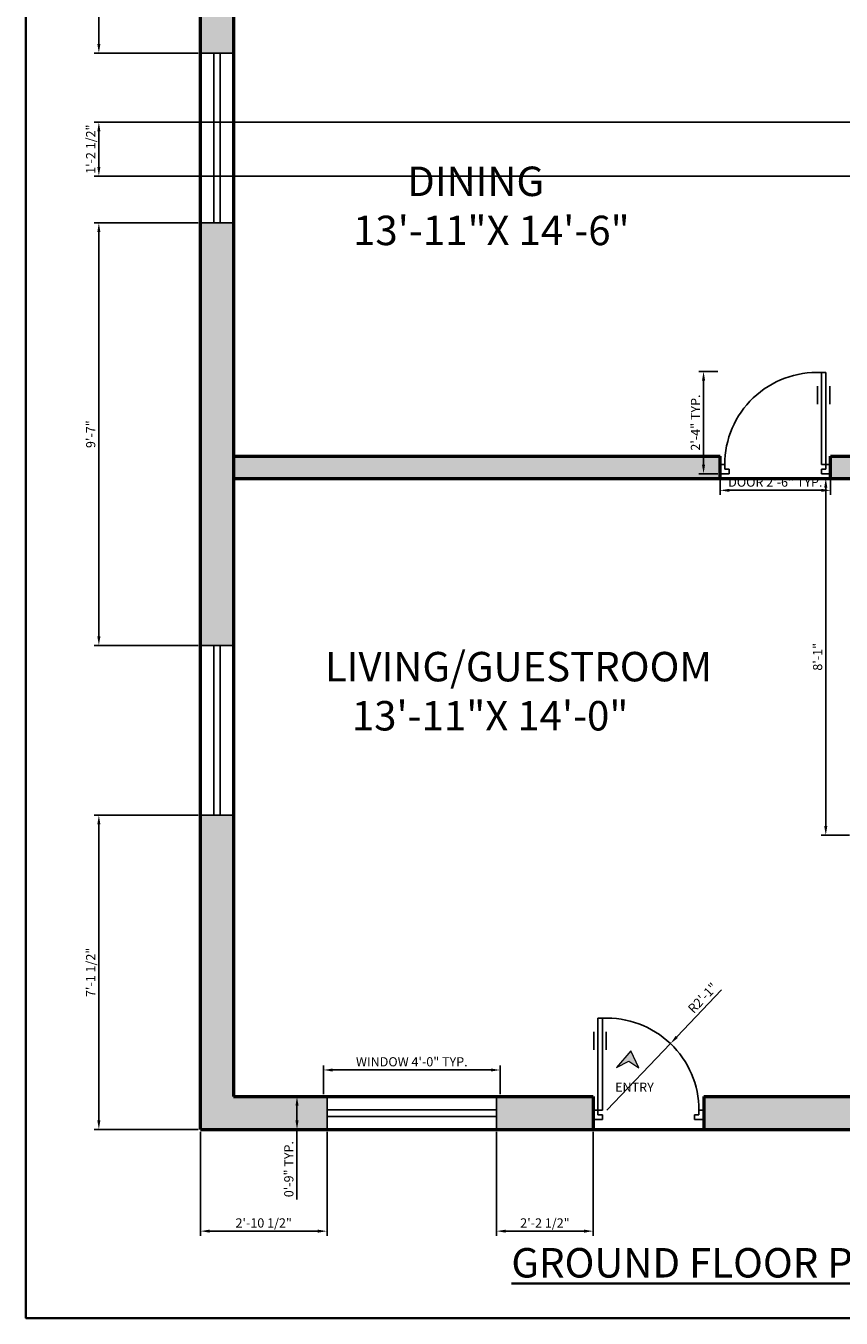
# Model space of a CAD drawing. Units: inches. Extents: x -36 to 398, y -51 to 516.
# Tile 1 of 3: x -36 to 186, y -51 to 300. Entities that reach past the tile are written whole.
import ezdxf

# ---------------------------------------------------------------- set-up
doc = ezdxf.new("R2010")
doc.units = ezdxf.units.IN
doc.header["$PDMODE"] = 34
for name, color, linetype, lineweight in [('A-ANNO-DIMS', 2, 'Continuous', 18), ('A-ANNO-SYMB', 7, 'Continuous', 18), ('A-ANNO-SYMB-PATT', 8, 'Continuous', 13), ('A-ANNO-TEXT', 7, 'Continuous', 18), ('A-ANNO-TTLB', 7, 'Continuous', 35), ('A-AREA-IDEN', 7, 'Continuous', 25), ('A-DOOR', 170, 'Continuous', 25), ('WALL', 7, 'Continuous', 50), ('WINDOW', 5, 'Continuous', 25)]:
    doc.layers.add(name, color=color, linetype=linetype, lineweight=lineweight)
doc.layers.add('A-WALL-PATT', color=251, linetype='Continuous', lineweight=13, true_color=0x636466)
doc.styles.get("Standard").update_dxf_attribs({"font": 'arial.ttf'})
doc.dimstyles.new('ISO-25', dxfattribs={"dimtxt": 2.5, "dimasz": 2.5, "dimexe": 1.25, "dimexo": 0.625, "dimtad": 1, "dimdec": 1, "dimlunit": 3, "dimtxsty": 'Standard', "dimcen": 2.5, "dimadec": 0, "dimazin": 0, "dimtfac": 1, "dimtdec": 1, "dimtmove": 0, "dimatfit": 3, "dimfxl": 1, "dimarcsym": 0})

# ---------------------------------------------------------------- blocks, each defined once
blk = doc.blocks.new('WD_00_X1')
for p, q in [((-0.5, 0.5), (0.5, 0.5)), ((-0.48, 0.5), (-0.48, -0.5)), ((0.48, 0.5), (0.48, -0.5)), ((0.48, 0.1), (-0.48, 0.1)), ((0.48, -0.1), (-0.48, -0.1)), ((-0.5, -0.5), (0.5, -0.5))]:
    blk.add_line(p, q)
blk = doc.blocks.new('DR_UKF1')
for p, q in [((-0.458, 0.042), (-0.458, 0.875)), ((-0.458, 0.875), (-0.417, 0.875)), ((-0.417, 0.875), (-0.417, 0.042)), ((-0.494, 0.751), (-0.494, 0.59)), ((-0.381, 0.751), (-0.381, 0.59)), ((-0.5, -0.042), (-0.5, 0.042)), ((-0.5, 0.042), (-0.458, 0.042)), ((-0.417, 0.042), (-0.458, 0.042)), ((-0.458, 0.042), (-0.458, 0)), ((-0.458, 0), (-0.417, 0)), ((-0.417, 0), (-0.417, -0.042)), ((0.417, 0), (0.417, -0.042)), ((0.458, 0), (0.417, 0)), ((0.458, 0.042), (0.458, 0)), ((0.5, 0.042), (0.458, 0.042)), ((0.5, -0.042), (0.5, 0.042)), ((-0.417, -0.042), (-0.5, -0.042)), ((-0.5, -0.042), (-0.5, -0.042)), ((0.417, -0.042), (0.5, -0.042)), ((0.5, -0.042), (0.5, -0.042))]:
    blk.add_line(p, q)
blk.add_arc((-0.375, 0.043), 0.833, 359.9283, 92.866)
blk = doc.blocks.new('*D14')
at = {"layer": 'A-ANNO-DIMS', "color": 0, "lineweight": -2, "transparency": 16777216}
for p, q in [((188.09, 176.98), (180.39, 176.98)), ((181.64, 174.48), (181.64, 82.48)), ((188.09, 79.98), (180.39, 79.98))]:
    blk.add_line(p, q, dxfattribs=at)
at = {"layer": 'A-ANNO-DIMS', "color": 0, "transparency": 16777216}
for points in [[(181.23, 174.48), (182.06, 174.48), (181.64, 176.98)], [(181.23, 82.48), (182.06, 82.48), (181.64, 79.98)]]:
    blk.add_solid(points, dxfattribs=at)
at = {"layer": 'Defpoints', "color": 0, "transparency": 16777216}
for p in [(188.71, 176.98), (181.64, 79.98), (188.71, 79.98)]:
    blk.add_point(p, dxfattribs=at)
at = {"layer": 'A-ANNO-DIMS', "color": 0, "transparency": 16777216, "insert": (179.74, 128.48), "char_height": 2.5, "attachment_point": 5, "rotation": 90}
blk.add_mtext('8\'-1"', dxfattribs=at)
blk = doc.blocks.new('*D18')
at = {"layer": 'A-ANNO-DIMS', "color": 0, "lineweight": -2, "transparency": 16777216}
for p, q in [((45.15, 9.6), (45.15, 17.43)), ((90.65, 16.18), (47.65, 16.18)), ((93.15, 9.6), (93.15, 17.43))]:
    blk.add_line(p, q, dxfattribs=at)
at = {"layer": 'A-ANNO-DIMS', "color": 0, "transparency": 16777216}
for points in [[(47.65, 16.59), (47.65, 15.76), (45.15, 16.18)], [(90.65, 16.59), (90.65, 15.76), (93.15, 16.18)]]:
    blk.add_solid(points, dxfattribs=at)
at = {"layer": 'Defpoints', "color": 0, "transparency": 16777216}
for p in [(45.15, 16.18), (45.15, 8.98), (93.15, 8.98)]:
    blk.add_point(p, dxfattribs=at)
at = {"layer": 'A-ANNO-DIMS', "color": 0, "transparency": 16777216, "insert": (69.15, 18.09), "char_height": 2.5, "attachment_point": 5}
blk.add_mtext('WINDOW 4\'-0" TYP.', dxfattribs=at)
blk = doc.blocks.new('*D19')
at = {"layer": 'A-ANNO-DIMS', "color": 0, "lineweight": -2, "transparency": 16777216}
for p, q in [((44.53, 8.98), (36.7, 8.98)), ((37.95, 6.48), (37.95, 2.48)), ((44.53, -0.02), (36.7, -0.02)), ((37.95, -0.02), (37.95, -19.01))]:
    blk.add_line(p, q, dxfattribs=at)
at = {"layer": 'A-ANNO-DIMS', "color": 0, "transparency": 16777216}
for points in [[(37.54, 6.48), (38.37, 6.48), (37.95, 8.98)], [(37.54, 2.48), (38.37, 2.48), (37.95, -0.02)]]:
    blk.add_solid(points, dxfattribs=at)
at = {"layer": 'Defpoints', "color": 0, "transparency": 16777216}
for p in [(45.15, 8.98), (37.95, -0.02), (45.15, -0.02)]:
    blk.add_point(p, dxfattribs=at)
at = {"layer": 'A-ANNO-DIMS', "color": 0, "transparency": 16777216, "insert": (36.05, -10.77), "char_height": 2.5, "attachment_point": 5, "rotation": 90}
blk.add_mtext('0\'-9" TYP.', dxfattribs=at)
blk = doc.blocks.new('*D22')
at = {"layer": 'A-ANNO-DIMS', "color": 0, "lineweight": -2, "transparency": 16777216}
for p, q in [((152.93, 177.6), (152.93, 172.48)), ((182.93, 177.6), (182.93, 172.48)), ((180.43, 173.73), (155.43, 173.73))]:
    blk.add_line(p, q, dxfattribs=at)
at = {"layer": 'A-ANNO-DIMS', "color": 0, "transparency": 16777216}
for points in [[(155.43, 174.14), (155.43, 173.31), (152.93, 173.73)], [(180.43, 174.14), (180.43, 173.31), (182.93, 173.73)]]:
    blk.add_solid(points, dxfattribs=at)
at = {"layer": 'Defpoints', "color": 0, "transparency": 16777216}
for p in [(152.93, 178.23), (182.93, 178.23), (152.93, 173.73)]:
    blk.add_point(p, dxfattribs=at)
at = {"layer": 'A-ANNO-DIMS', "color": 0, "transparency": 16777216, "insert": (167.93, 175.64), "char_height": 2.5, "attachment_point": 5}
blk.add_mtext('DOOR 2\'-6" TYP.', dxfattribs=at)
blk = doc.blocks.new('*D23')
at = {"layer": 'A-ANNO-DIMS', "color": 0, "lineweight": -2, "transparency": 16777216}
for p, q in [((152.3, 206.07), (147.18, 206.07)), ((148.43, 180.73), (148.43, 203.57)), ((152.3, 178.23), (147.18, 178.23))]:
    blk.add_line(p, q, dxfattribs=at)
at = {"layer": 'A-ANNO-DIMS', "color": 0, "transparency": 16777216}
for points in [[(148.01, 203.57), (148.85, 203.57), (148.43, 206.07)], [(148.01, 180.73), (148.85, 180.73), (148.43, 178.23)]]:
    blk.add_solid(points, dxfattribs=at)
at = {"layer": 'Defpoints', "color": 0, "transparency": 16777216}
for p in [(148.43, 206.07), (152.93, 206.07), (152.93, 178.23)]:
    blk.add_point(p, dxfattribs=at)
at = {"layer": 'A-ANNO-DIMS', "color": 0, "transparency": 16777216, "insert": (146.55, 192.15), "char_height": 2.5, "attachment_point": 5, "rotation": 90}
blk.add_mtext('2\'-4" TYP.', dxfattribs=at)
blk = doc.blocks.new('*D35')
at = {"layer": 'A-ANNO-DIMS', "color": 0, "lineweight": -2, "transparency": 16777216}
for p, q in [((11.71, -0.65), (11.71, -28.87)), ((46.11, -0.65), (46.11, -28.87)), ((14.21, -27.62), (43.61, -27.62))]:
    blk.add_line(p, q, dxfattribs=at)
at = {"layer": 'A-ANNO-DIMS', "color": 0, "transparency": 16777216}
for points in [[(14.21, -27.21), (14.21, -28.04), (11.71, -27.62)], [(43.61, -27.21), (43.61, -28.04), (46.11, -27.62)]]:
    blk.add_solid(points, dxfattribs=at)
at = {"layer": 'Defpoints', "color": 0, "transparency": 16777216}
for p in [(11.71, -0.02), (46.11, -0.02), (46.11, -27.62)]:
    blk.add_point(p, dxfattribs=at)
at = {"layer": 'A-ANNO-DIMS', "color": 0, "transparency": 16777216, "insert": (28.91, -25.71), "char_height": 2.5, "attachment_point": 5}
blk.add_mtext('2\'-10 1/2"', dxfattribs=at)
blk = doc.blocks.new('*D36')
at = {"layer": 'A-ANNO-DIMS', "color": 0, "lineweight": -2, "transparency": 16777216}
for p, q in [((92.19, -0.65), (92.19, -28.87)), ((118.46, -0.65), (118.46, -28.87)), ((94.69, -27.62), (115.96, -27.62))]:
    blk.add_line(p, q, dxfattribs=at)
at = {"layer": 'A-ANNO-DIMS', "color": 0, "transparency": 16777216}
for points in [[(94.69, -27.21), (94.69, -28.04), (92.19, -27.62)], [(115.96, -27.21), (115.96, -28.04), (118.46, -27.62)]]:
    blk.add_solid(points, dxfattribs=at)
at = {"layer": 'Defpoints', "color": 0, "transparency": 16777216}
for p in [(92.19, -0.02), (118.46, -0.02), (118.46, -27.62)]:
    blk.add_point(p, dxfattribs=at)
at = {"layer": 'A-ANNO-DIMS', "color": 0, "transparency": 16777216, "insert": (105.33, -25.71), "char_height": 2.5, "attachment_point": 5}
blk.add_mtext('2\'-2 1/2"', dxfattribs=at)
blk = doc.blocks.new('*D37')
at = {"layer": 'A-ANNO-DIMS', "color": 0, "lineweight": -2, "transparency": 16777216}
for p, q in [((11.09, 85.44), (-17.14, 85.44)), ((-15.89, 2.48), (-15.89, 82.94)), ((11.09, -0.02), (-17.14, -0.02))]:
    blk.add_line(p, q, dxfattribs=at)
at = {"layer": 'A-ANNO-DIMS', "color": 0, "transparency": 16777216}
for points in [[(-16.3, 82.94), (-15.47, 82.94), (-15.89, 85.44)], [(-16.3, 2.48), (-15.47, 2.48), (-15.89, -0.02)]]:
    blk.add_solid(points, dxfattribs=at)
at = {"layer": 'Defpoints', "color": 0, "transparency": 16777216}
for p in [(-15.89, 85.44), (11.71, 85.44), (11.71, -0.02)]:
    blk.add_point(p, dxfattribs=at)
at = {"layer": 'A-ANNO-DIMS', "color": 0, "transparency": 16777216, "insert": (-17.8, 42.71), "char_height": 2.5, "attachment_point": 5, "rotation": 90}
blk.add_mtext('7\'-1 1/2"', dxfattribs=at)
blk = doc.blocks.new('*D38')
at = {"layer": 'A-ANNO-DIMS', "color": 0, "lineweight": -2, "transparency": 16777216}
for p, q in [((11.09, 246.46), (-17.14, 246.46)), ((-15.89, 134.02), (-15.89, 243.96)), ((11.09, 131.52), (-17.14, 131.52))]:
    blk.add_line(p, q, dxfattribs=at)
at = {"layer": 'A-ANNO-DIMS', "color": 0, "transparency": 16777216}
for points in [[(-16.3, 243.96), (-15.47, 243.96), (-15.89, 246.46)], [(-16.3, 134.02), (-15.47, 134.02), (-15.89, 131.52)]]:
    blk.add_solid(points, dxfattribs=at)
at = {"layer": 'Defpoints', "color": 0, "transparency": 16777216}
for p in [(-15.89, 246.46), (11.71, 246.46), (11.71, 131.52)]:
    blk.add_point(p, dxfattribs=at)
at = {"layer": 'A-ANNO-DIMS', "color": 0, "transparency": 16777216, "insert": (-17.79, 188.99), "char_height": 2.5, "attachment_point": 5, "rotation": 90}
blk.add_mtext('9\'-7"', dxfattribs=at)
blk = doc.blocks.new('*D39')
at = {"layer": 'A-ANNO-DIMS', "color": 0, "lineweight": -2, "transparency": 16777216}
for p, q in [((11.09, 367.07), (-17.14, 367.07)), ((-15.89, 295.04), (-15.89, 364.57)), ((11.09, 292.54), (-17.14, 292.54))]:
    blk.add_line(p, q, dxfattribs=at)
at = {"layer": 'A-ANNO-DIMS', "color": 0, "transparency": 16777216}
for points in [[(-16.3, 364.57), (-15.47, 364.57), (-15.89, 367.07)], [(-16.3, 295.04), (-15.47, 295.04), (-15.89, 292.54)]]:
    blk.add_solid(points, dxfattribs=at)
at = {"layer": 'Defpoints', "color": 0, "transparency": 16777216}
for p in [(-15.89, 367.07), (11.71, 367.07), (11.71, 292.54)]:
    blk.add_point(p, dxfattribs=at)
at = {"layer": 'A-ANNO-DIMS', "color": 0, "transparency": 16777216, "insert": (-17.8, 329.81), "char_height": 2.5, "attachment_point": 5, "rotation": 90}
blk.add_mtext('6\'-2 1/2"', dxfattribs=at)
blk = doc.blocks.new('*D48')
at = {"layer": 'A-ANNO-DIMS', "color": 0, "lineweight": -2, "transparency": 16777216}
for p, q in [((326.09, 273.8), (-17.14, 273.8)), ((-15.89, 271.3), (-15.89, 261.6)), ((326.09, 259.1), (-17.14, 259.1))]:
    blk.add_line(p, q, dxfattribs=at)
at = {"layer": 'A-ANNO-DIMS', "color": 0, "transparency": 16777216}
for points in [[(-16.3, 271.3), (-15.47, 271.3), (-15.89, 273.8)], [(-16.3, 261.6), (-15.47, 261.6), (-15.89, 259.1)]]:
    blk.add_solid(points, dxfattribs=at)
at = {"layer": 'Defpoints', "color": 0, "transparency": 16777216}
for p in [(326.71, 273.8), (-15.89, 259.1), (326.71, 259.1)]:
    blk.add_point(p, dxfattribs=at)
at = {"layer": 'A-ANNO-DIMS', "color": 0, "transparency": 16777216, "insert": (-17.8, 266.45), "char_height": 2.5, "attachment_point": 5, "rotation": 90}
blk.add_mtext('1\'-2 1/2"', dxfattribs=at)
blk = doc.blocks.new('*D51')
at = {"layer": 'A-ANNO-DIMS', "color": 0, "lineweight": -2, "transparency": 16777216}
for p, q in [((153.33, 37.96), (141.16, 25.18)), ((122.19, 5.27), (139.44, 23.37))]:
    blk.add_line(p, q, dxfattribs=at)
at = {"layer": 'A-ANNO-DIMS', "color": 0, "transparency": 16777216}
blk.add_solid([(140.86, 25.47), (141.46, 24.89), (139.44, 23.37)], dxfattribs=at)
at = {"layer": 'Defpoints', "color": 0, "transparency": 16777216}
for p in [(139.44, 23.37), (122.19, 5.27)]:
    blk.add_point(p, dxfattribs=at)
at = {"layer": 'A-ANNO-DIMS', "color": 0, "transparency": 16777216, "insert": (148.42, 35.53), "char_height": 2.5, "attachment_point": 5, "rotation": 46.3968}
blk.add_mtext('R2\'-1"', dxfattribs=at)

msp = doc.modelspace()

# ---------------------------------------------------------------- hatches: boundary and pattern name
at = {"layer": 'A-ANNO-SYMB-PATT'}
h = msp.add_hatch(color=256, dxfattribs=at)
h.dxf.hatch_style = 1
h.paths.add_polyline_path([(128.63, 21.38), (124.8, 16.86), (128.1, 18.56), (130.82, 16.8)])
at = {"layer": 'A-WALL-PATT'}
h = msp.add_hatch(color=256, dxfattribs=at)
h.dxf.hatch_style = 1
h.paths.add_polyline_path([(335.71, 155.4), (326.71, 155.4), (326.71, 154.44), (326.71, 50.65), (335.71, 50.65), (335.71, 51.01)])
h.paths.add_polyline_path([(335.71, 257.33), (326.71, 257.33), (326.71, 256.97), (326.71, 201.48), (335.71, 201.48), (335.71, 202.44)])
h.paths.add_polyline_path([(335.71, 33.37), (326.71, 33.37), (326.71, 33.01), (326.71, 8.98), (200.71, 8.98), (148.47, 8.98), (148.47, -0.02), (335.71, -0.02)])
h.paths.add_polyline_path([(118.44, 5.24), (118.46, 8.98), (92.19, 8.98), (92.19, -0.02), (93.15, -0.02), (118.46, -0.02), (118.46, 2.74), (118.44, 2.74)])
h.paths.add_polyline_path([(20.71, 85.44), (11.71, 85.44), (11.71, 84.48), (11.71, -0.02), (46.11, -0.02), (46.11, 8.98), (45.15, 8.98), (20.71, 8.98)])
h.paths.add_polyline_path([(20.71, 246.46), (11.71, 246.46), (11.71, 245.5), (11.71, 131.52), (20.71, 131.52), (20.71, 132.48)])
h.paths.add_polyline_path([(152.93, 182.98), (20.71, 182.98), (20.71, 176.98), (152.93, 176.98)])
h.paths.add_polyline_path([(188.71, 182.98), (182.93, 182.98), (182.93, 176.98), (188.71, 176.98)])
h.paths.add_polyline_path([(194.71, 224.98), (199.29, 224.98), (199.29, 230.98), (188.71, 230.98), (188.71, 79.98), (210.71, 79.98), (210.71, 80.98), (326.71, 80.98), (326.71, 85.98), (194.71, 85.98)])
h.paths.add_polyline_path([(326.71, 230.98), (229.41, 230.98), (229.41, 224.98), (326.71, 224.98)], flags=0)
h.paths.add_polyline_path([(242.71, 276.58), (236.71, 276.58), (236.71, 230.98), (242.71, 230.98)])
h.paths.add_polyline_path([(326.71, 302.98), (194.71, 302.98), (194.71, 310.64), (188.71, 310.64), (188.71, 296.98), (326.71, 296.98)])
h.paths.add_polyline_path([(242.71, 296.98), (236.71, 296.98), (236.71, 294.58), (242.71, 294.58)])
h.paths.add_polyline_path([(194.71, 434.98), (188.71, 434.98), (188.71, 340.61), (191.4, 340.61), (191.4, 340.64), (193.9, 340.64), (194.71, 340.61)])
h.paths.add_polyline_path([(335.71, 443.98), (174.69, 443.98), (174.69, 434.98), (175.05, 434.98), (326.71, 434.98), (326.71, 384.97), (335.71, 384.97), (335.71, 385.93)])
h.paths.add_polyline_path([(335.71, 338.89), (326.71, 338.89), (326.71, 337.93), (326.71, 274.61), (335.71, 274.61), (335.71, 274.97)])
h.paths.add_polyline_path([(157.41, 443.98), (157.05, 443.98), (11.71, 443.98), (11.71, 413.15), (20.71, 413.15), (20.71, 414.11), (20.71, 434.98), (157.41, 434.98)])
h.paths.add_polyline_path([(20.71, 367.07), (11.71, 367.07), (11.71, 366.11), (11.71, 292.54), (20.71, 292.54), (20.71, 293.5)])

# ---------------------------------------------------------------- linework, layer by layer
at = {"layer": 'A-ANNO-SYMB'}
for p, q in [((128.63, 21.38), (124.8, 16.86)), ((130.82, 16.8), (128.63, 21.38)), ((124.8, 16.86), (128.1, 18.56)), ((128.1, 18.56), (130.82, 16.8))]:
    msp.add_line(p, q, dxfattribs=at)
at = {"layer": 'A-ANNO-TTLB'}
msp.add_lwpolyline([(-35.73, 515.75), (386.76, 515.75), (386.76, -51.27), (-35.73, -51.27)], close=True, dxfattribs=at)
at = {"layer": 'WALL'}
for p, q in [((11.71, -0.02), (11.71, 443.98)), ((20.71, 434.98), (20.71, 8.98)), ((20.71, 182.98), (152.93, 182.98)), ((152.93, 176.98), (152.93, 182.98)), ((182.93, 176.98), (182.93, 182.98)), ((182.93, 182.98), (188.71, 182.98)), ((20.71, 176.98), (188.71, 176.98)), ((20.71, 8.98), (118.46, 8.98)), ((118.46, 8.98), (118.46, -0.02)), ((148.47, 8.98), (148.47, -0.02)), ((148.47, 8.98), (326.71, 8.98)), ((11.71, -0.02), (335.71, -0.02))]:
    msp.add_line(p, q, dxfattribs=at)

# ---------------------------------------------------------------- block references
at = {"layer": 'A-DOOR', "xscale": -30, "yscale": 30, "zscale": 30, "rotation": 359.9999999999882}
msp.add_blockref('DR_UKF1', (167.93, 179.48), dxfattribs=at)
at = {"layer": 'A-DOOR', "xscale": 30, "yscale": 30, "zscale": 30}
msp.add_blockref('DR_UKF1', (133.44, 3.99), dxfattribs=at)
at = {"layer": 'WINDOW', "xscale": 48, "yscale": 9, "zscale": 48}
for p, rotation in [((16.21, 269.5), 89.99999999999999), ((16.21, 108.48), 89.99999999999999), ((69.15, 4.48), 180)]:
    msp.add_blockref('WD_00_X1', p, dxfattribs=dict(at, rotation=rotation))

# ---------------------------------------------------------------- texts
at = {"layer": 'A-ANNO-TEXT', "insert": (124.41, 12.75), "char_height": 2.5, "attachment_point": 1}
msp.add_mtext_dynamic_manual_height_columns('ENTRY', width=14.657, gutter_width=12.5, heights=[0], dxfattribs=at)
at = {"layer": 'A-ANNO-TTLB', "insert": (96.2, -32.22), "char_height": 8.0065, "attachment_point": 1}
msp.add_mtext_dynamic_manual_height_columns('{\\fArial|b1|i0|c0|p34;\\LGROUND FLOOR PLAN}', width=139.8375, gutter_width=40.03, heights=[0], dxfattribs=at)
at = {"layer": 'A-AREA-IDEN', "char_height": 8.0065, "attachment_point": 1}
for s, insert in [('      DINING\\P13\'-11"X 14\'-6"', (53.2, 261.72)), ('LIVING/GUESTROOM\\P   13\'-11"X 14\'-0"', (45.52, 129.81))]:
    msp.add_mtext_dynamic_manual_height_columns(s, width=96.1834, gutter_width=40.03, heights=[0], dxfattribs=dict(at, insert=insert))

# ---------------------------------------------------------------- dimensions: what is measured, and where the dimension line sits
at = {"layer": 'A-ANNO-DIMS'}
for base, p1, p2, override, picture, middle in [((-15.89, 367.07), (11.71, 292.54), (11.71, 367.07), {"dimdec": 1, "dimlfac": 1, "dimrnd": 0, "dimzin": 1, "dimdsep": 46, "dimlunit": 4, "dimfrac": 2}, '*D39', (-17.8, 329.81)), ((-15.89, 259.1), (326.71, 273.8), (326.71, 259.1), {"dimdec": 1, "dimlfac": 1, "dimrnd": 0, "dimzin": 1, "dimdsep": 46, "dimlunit": 4, "dimfrac": 2}, '*D48', (-17.8, 266.45)), ((-15.89, 246.46), (11.71, 131.52), (11.71, 246.46), {"dimdec": 1, "dimlfac": 1, "dimrnd": 0, "dimzin": 1, "dimdsep": 46, "dimlunit": 4, "dimfrac": 2}, '*D38', (-17.79, 188.99)), ((181.64, 79.98), (188.71, 176.98), (188.71, 79.98), {"dimclrd": 0, "dimclre": 0, "dimclrt": 0}, '*D14', (179.74, 128.48)), ((-15.89, 85.44), (11.71, -0.02), (11.71, 85.44), {"dimdec": 1, "dimlfac": 1, "dimrnd": 0, "dimzin": 1, "dimdsep": 46, "dimlunit": 4, "dimfrac": 2}, '*D37', (-17.8, 42.71))]:
    dim = msp.add_linear_dim(base=base, p1=p1, p2=p2, angle=90, dimstyle='ISO-25', override=override, dxfattribs=at)
    dim.commit()
    dim.dimension.update_dxf_attribs({"geometry": picture, "text_midpoint": middle})
for base, p1, p2, angle, text, picture, middle in [((148.43, 206.07), (152.93, 178.23), (152.93, 206.07), 90, '<> TYP.', '*D23', (146.55, 192.15)), ((152.93, 173.73), (182.93, 178.23), (152.93, 178.23), 180, 'DOOR <> TYP.', '*D22', (167.93, 175.64)), ((45.15, 16.18), (93.15, 8.98), (45.15, 8.98), 180, 'WINDOW <> TYP.', '*D18', (69.15, 18.09)), ((37.95, -0.02), (45.15, 8.98), (45.15, -0.02), 270, '<> TYP.', '*D19', (36.05, -10.77))]:
    dim = msp.add_linear_dim(base=base, p1=p1, p2=p2, angle=angle, text=text, dimstyle='ISO-25', override={"dimdec": 1, "dimlfac": 1, "dimrnd": 0, "dimzin": 1, "dimdsep": 46, "dimlunit": 4, "dimfrac": 2}, dxfattribs=at)
    dim.commit()
    dim.dimension.update_dxf_attribs({"geometry": picture, "text_midpoint": middle})
dim = msp.add_radius_dim(center=(122.19, 5.27), mpoint=(139.44, 23.37), dimstyle='ISO-25', override={"dimdec": 1, "dimlfac": 1, "dimrnd": 0, "dimzin": 1, "dimdsep": 46, "dimlunit": 4, "dimfrac": 2}, dxfattribs=at)
dim.commit()
dim.dimension.update_dxf_attribs({"geometry": '*D51', "text_midpoint": (149.78, 34.23), "dimtype": 164})
for base, p1, p2, picture, middle in [((46.11, -27.62), (11.71, -0.02), (46.11, -0.02), '*D35', (28.91, -25.71)), ((118.46, -27.62), (92.19, -0.02), (118.46, -0.02), '*D36', (105.33, -25.71))]:
    dim = msp.add_linear_dim(base=base, p1=p1, p2=p2, dimstyle='ISO-25', override={"dimdec": 1, "dimlfac": 1, "dimrnd": 0, "dimzin": 1, "dimdsep": 46, "dimlunit": 4, "dimfrac": 2}, dxfattribs=at)
    dim.commit()
    dim.dimension.update_dxf_attribs({"geometry": picture, "text_midpoint": middle})

doc.saveas('drawing.dxf')
